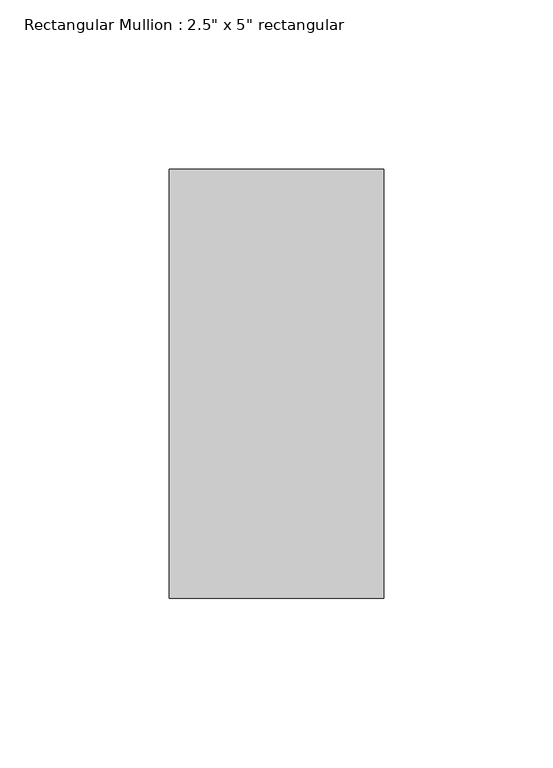
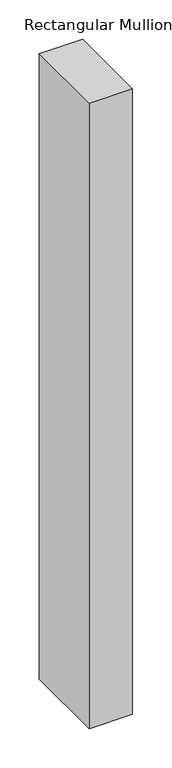
"""IFC4 building model written with IfcOpenShell, lengths in millimetres: member geometry."""

from ifc_helpers import new_model, si_unit, frame, origin, place, context, project, spatial, polyline, outline, extrude, source, transform, mapped, element, save


def member_88aa5c81(model_context):
    return source(origin(), model_context, "Body", "SweptSolid", [
        extrude(outline(polyline([(31.75, 63.5), (31.75, -63.5), (-31.75, -63.5), (-31.75, 63.5), (31.75, 63.5)])), frame((0.0, 0.0, -971.55), z_axis=(0.0, 0.0, 1.0), x_axis=(1.0, 0.0, 0.0)), (0.0, 0.0, 1.0), 971.55),
    ])


if __name__ == "__main__":
    model = new_model("IFC4")
    model_context = context("Model", 3, world=origin())
    ifc_project = project(units=[si_unit("LENGTHUNIT", "METRE", prefix="MILLI")], contexts=[model_context])
    site = spatial("IfcSite", under=ifc_project)
    building = spatial("IfcBuilding", under=site)
    placement = place(None, origin())
    member_shape = member_88aa5c81(model_context)
    element("IfcMember", 1, ObjectType="Rectangular Mullion : 2.5\" x 5\" rectangular", at=placement, inside=building, context=model_context, shape_type="MappedRepresentation", body=[
        mapped(member_shape, transform((0.0, 0.0, 0.0), x_axis=(1.0, 0.0, 0.0), y_axis=(0.0, 1.0, 0.0), z_axis=(0.0, 0.0, 1.0))),
    ])
    save(model, "model.ifc")

# Revit data of these elements
# Type "Rectangular Mullion : 2.5\" x 5\" rectangular"
#   built-in parameter 1007304 = 0.416667 (stored number, unit not read)
#   built-in parameter 1007301 = 0.104167 (stored number, unit not read)
#   built-in parameter 1007300 = 0.104167 (stored number, unit not read)
# Element 1 (IfcMember, "Rectangular Mullion : 2.5\" x 5\" rectangular")
#   Materials on its faces: "Aluminum"
# Materials
#   "Aluminum": class "Metal", colour RGB 247 247 247, transparency 0, Description = "Aluminum 6061", Cost = 0
